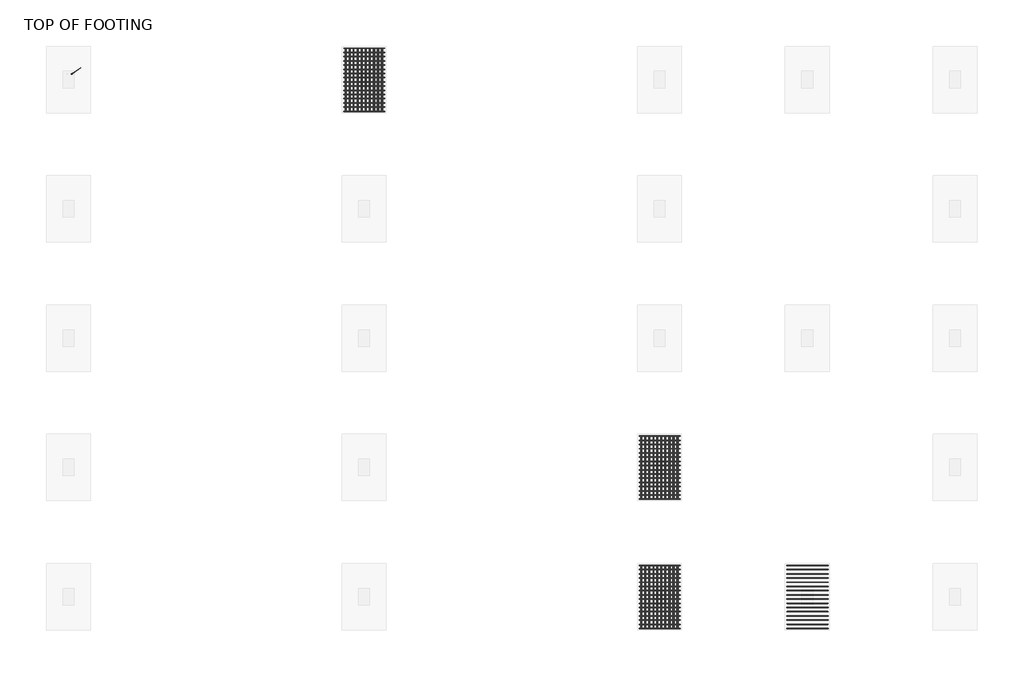
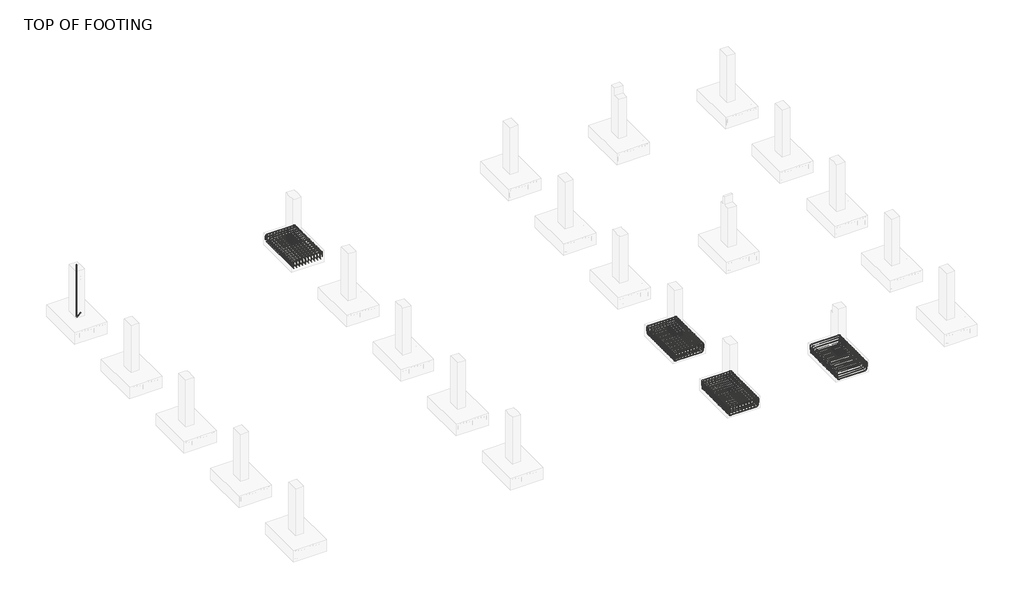
# One storey, part 5 of 8: 14 reinforcing bars.
"""IFC4 building model written with IfcOpenShell, lengths in millimetres."""

from ifc_helpers import new_model, si_unit, point, frame, origin, place, context, project, spatial, polyline, circle_curve, trimmed, segment, composite_curve, source, transform, mapped, element, save
from ifc_brep_helpers import swept_disk

model = new_model("IFC4")

# Units and contexts
model_context = context("Model", 3, world=origin())
ifc_project = project(units=[si_unit("LENGTHUNIT", "METRE", prefix="MILLI")], contexts=[model_context])

# Site, building, storey
site = spatial("IfcSite", under=ifc_project)
building = spatial("IfcBuilding", under=site)
storey = spatial("IfcBuildingStorey", under=building, Name="TOP OF FOOTING", Elevation=-1828.8)

# Reinforcing bars
placement = place(None, origin())
element("IfcReinforcingBar", 1, at=placement, inside=storey, context=model_context, shape_type="SolidModel", body=[
    swept_disk(composite_curve([segment(polyline([(-11755.8874017, 15924.2508557, -40.0), (-11755.8874017, 15924.2508557, -2055.5685723)]), True, "CONTINUOUS"), segment(trimmed(circle_curve(frame((-11717.9197045, 15950.8361235, -2055.5685723), z_axis=(0.5735764363510459, -0.819152044288992, 0.0), x_axis=(-37.96769719999975, -26.5852677999992, 0.0)), 46.35), [point((-11755.8874017, 15924.2508557, -2055.5685723))], [point((-11717.9197045, 15950.8361235, -2101.9185723))], True, "CARTESIAN"), True, "CONTINUOUS"), segment(polyline([(-11717.9197045, 15950.8361235, -2101.9185723), (-11506.0932621, 16099.1585953, -2101.9185723)]), True, "CONTINUOUS")], self_intersect=False), 6.35),
])
reinforcing_bar_shape = source(origin(), model_context, "Body", "SolidModel", [
    swept_disk(composite_curve([segment(polyline([(-4384.3374017, 16626.3508557, -2068.8), (-4384.3374017, 16626.3508557, -1921.5)]), True, "CONTINUOUS"), segment(trimmed(circle_curve(frame((-4337.9874017, 16626.3508557, -1921.5), z_axis=(0.0, 1.0, 0.0), x_axis=(-46.349999999999454, 0.0, 0.0)), 46.35), [point((-4384.3374017, 16626.3508557, -1921.5))], [point((-4337.9874017, 16626.3508557, -1875.15))], True, "CARTESIAN"), True, "CONTINUOUS"), segment(polyline([(-4337.9874017, 16626.3508557, -1875.15), (-3323.3874017, 16626.3508557, -1875.15)]), True, "CONTINUOUS"), segment(trimmed(circle_curve(frame((-3323.3874017, 16626.3508557, -1921.5), z_axis=(0.0, 1.0, 0.0), x_axis=(0.0, 0.0, 46.34999999999991)), 46.35), [point((-3323.3874017, 16626.3508557, -1875.15))], [point((-3277.0374017, 16626.3508557, -1921.5))], True, "CARTESIAN"), True, "CONTINUOUS"), segment(polyline([(-3277.0374017, 16626.3508557, -1921.5), (-3277.0374017, 16626.3508557, -2068.8)]), True, "CONTINUOUS")], self_intersect=False), 6.35),
])
element("IfcReinforcingBar", 2, at=placement, inside=storey, context=model_context, shape_type="MappedRepresentation", body=[
    mapped(reinforcing_bar_shape, transform((0.0, 0.0, 0.0), x_axis=(1.0, 0.0, 0.0), y_axis=(0.0, 1.0, 0.0), z_axis=(0.0, 0.0, 1.0))),
    mapped(reinforcing_bar_shape, transform((0.0, -113.82, 0.0), x_axis=(1.0, 0.0, 0.0), y_axis=(0.0, 1.0, 0.0), z_axis=(0.0, 0.0, 1.0))),
    mapped(reinforcing_bar_shape, transform((0.0, -227.64, 0.0), x_axis=(1.0, 0.0, 0.0), y_axis=(0.0, 1.0, 0.0), z_axis=(0.0, 0.0, 1.0))),
    mapped(reinforcing_bar_shape, transform((0.0, -341.46, 0.0), x_axis=(1.0, 0.0, 0.0), y_axis=(0.0, 1.0, 0.0), z_axis=(0.0, 0.0, 1.0))),
    mapped(reinforcing_bar_shape, transform((0.0, -455.28, 0.0), x_axis=(1.0, 0.0, 0.0), y_axis=(0.0, 1.0, 0.0), z_axis=(0.0, 0.0, 1.0))),
    mapped(reinforcing_bar_shape, transform((0.0, -569.1, 0.0), x_axis=(1.0, 0.0, 0.0), y_axis=(0.0, 1.0, 0.0), z_axis=(0.0, 0.0, 1.0))),
    mapped(reinforcing_bar_shape, transform((0.0, -682.92, 0.0), x_axis=(1.0, 0.0, 0.0), y_axis=(0.0, 1.0, 0.0), z_axis=(0.0, 0.0, 1.0))),
    mapped(reinforcing_bar_shape, transform((0.0, -796.74, 0.0), x_axis=(1.0, 0.0, 0.0), y_axis=(0.0, 1.0, 0.0), z_axis=(0.0, 0.0, 1.0))),
    mapped(reinforcing_bar_shape, transform((0.0, -910.56, 0.0), x_axis=(1.0, 0.0, 0.0), y_axis=(0.0, 1.0, 0.0), z_axis=(0.0, 0.0, 1.0))),
    mapped(reinforcing_bar_shape, transform((0.0, -1024.38, 0.0), x_axis=(1.0, 0.0, 0.0), y_axis=(0.0, 1.0, 0.0), z_axis=(0.0, 0.0, 1.0))),
    mapped(reinforcing_bar_shape, transform((0.0, -1138.2, 0.0), x_axis=(1.0, 0.0, 0.0), y_axis=(0.0, 1.0, 0.0), z_axis=(0.0, 0.0, 1.0))),
    mapped(reinforcing_bar_shape, transform((0.0, -1252.02, 0.0), x_axis=(1.0, 0.0, 0.0), y_axis=(0.0, 1.0, 0.0), z_axis=(0.0, 0.0, 1.0))),
    mapped(reinforcing_bar_shape, transform((0.0, -1365.84, 0.0), x_axis=(1.0, 0.0, 0.0), y_axis=(0.0, 1.0, 0.0), z_axis=(0.0, 0.0, 1.0))),
    mapped(reinforcing_bar_shape, transform((0.0, -1479.66, 0.0), x_axis=(1.0, 0.0, 0.0), y_axis=(0.0, 1.0, 0.0), z_axis=(0.0, 0.0, 1.0))),
    mapped(reinforcing_bar_shape, transform((0.0, -1593.48, 0.0), x_axis=(1.0, 0.0, 0.0), y_axis=(0.0, 1.0, 0.0), z_axis=(0.0, 0.0, 1.0))),
    mapped(reinforcing_bar_shape, transform((0.0, -1707.3, 0.0), x_axis=(1.0, 0.0, 0.0), y_axis=(0.0, 1.0, 0.0), z_axis=(0.0, 0.0, 1.0))),
])
reinforcing_bar_2_shape = source(origin(), model_context, "Body", "SolidModel", [
    swept_disk(composite_curve([segment(polyline([(-4339.592709, 16632.7008557, -2155.1176129), (-4339.592709, 14912.7008557, -2155.1176129)]), True, "CONTINUOUS")], self_intersect=False), 6.35),
])
element("IfcReinforcingBar", 3, at=placement, inside=storey, context=model_context, shape_type="MappedRepresentation", body=[
    mapped(reinforcing_bar_2_shape, transform((0.0, 0.0, 0.0), x_axis=(1.0, 0.0, 0.0), y_axis=(0.0, 1.0, 0.0), z_axis=(0.0, 0.0, 1.0))),
    mapped(reinforcing_bar_2_shape, transform((111.602188, 0.0, 0.0), x_axis=(1.0, 0.0, 0.0), y_axis=(0.0, 1.0, 0.0), z_axis=(0.0, 0.0, 1.0))),
    mapped(reinforcing_bar_2_shape, transform((223.2043759, 0.0, 0.0), x_axis=(1.0, 0.0, 0.0), y_axis=(0.0, 1.0, 0.0), z_axis=(0.0, 0.0, 1.0))),
    mapped(reinforcing_bar_2_shape, transform((334.8065639, 0.0, 0.0), x_axis=(1.0, 0.0, 0.0), y_axis=(0.0, 1.0, 0.0), z_axis=(0.0, 0.0, 1.0))),
    mapped(reinforcing_bar_2_shape, transform((446.4087519, 0.0, 0.0), x_axis=(1.0, 0.0, 0.0), y_axis=(0.0, 1.0, 0.0), z_axis=(0.0, 0.0, 1.0))),
    mapped(reinforcing_bar_2_shape, transform((558.0109398, 0.0, 0.0), x_axis=(1.0, 0.0, 0.0), y_axis=(0.0, 1.0, 0.0), z_axis=(0.0, 0.0, 1.0))),
    mapped(reinforcing_bar_2_shape, transform((669.6131278, 0.0, 0.0), x_axis=(1.0, 0.0, 0.0), y_axis=(0.0, 1.0, 0.0), z_axis=(0.0, 0.0, 1.0))),
    mapped(reinforcing_bar_2_shape, transform((781.2153158, 0.0, 0.0), x_axis=(1.0, 0.0, 0.0), y_axis=(0.0, 1.0, 0.0), z_axis=(0.0, 0.0, 1.0))),
    mapped(reinforcing_bar_2_shape, transform((892.8175037, 0.0, 0.0), x_axis=(1.0, 0.0, 0.0), y_axis=(0.0, 1.0, 0.0), z_axis=(0.0, 0.0, 1.0))),
    mapped(reinforcing_bar_2_shape, transform((1004.4196917, 0.0, 0.0), x_axis=(1.0, 0.0, 0.0), y_axis=(0.0, 1.0, 0.0), z_axis=(0.0, 0.0, 1.0))),
])
reinforcing_bar_3_shape = source(origin(), model_context, "Body", "SolidModel", [
    swept_disk(composite_curve([segment(polyline([(-3364.2651981, 16626.3508557, -2094.6521303), (-3364.2651981, 16626.3508557, -1947.3521303)]), True, "CONTINUOUS"), segment(trimmed(circle_curve(frame((-3364.2651981, 16580.0008557, -1947.3521303), z_axis=(1.0, 0.0, 0.0), x_axis=(0.0, 46.349999999998545, 0.0)), 46.35), [point((-3364.2651981, 16626.3508557, -1947.3521303))], [point((-3364.2651981, 16580.0008557, -1901.0021303))], True, "CARTESIAN"), True, "CONTINUOUS"), segment(polyline([(-3364.2651981, 16580.0008557, -1901.0021303), (-3364.2651981, 14965.4008557, -1901.0021303)]), True, "CONTINUOUS"), segment(trimmed(circle_curve(frame((-3364.2651981, 14965.4008557, -1947.3521303), z_axis=(1.0, 0.0, 0.0), x_axis=(0.0, 0.0, 46.34999999999991)), 46.35), [point((-3364.2651981, 14965.4008557, -1901.0021303))], [point((-3364.2651981, 14919.0508557, -1947.3521303))], True, "CARTESIAN"), True, "CONTINUOUS"), segment(polyline([(-3364.2651981, 14919.0508557, -1947.3521303), (-3364.2651981, 14919.0508557, -2094.6521303)]), True, "CONTINUOUS")], self_intersect=False), 6.35),
])
element("IfcReinforcingBar", 4, at=placement, inside=storey, context=model_context, shape_type="MappedRepresentation", body=[
    mapped(reinforcing_bar_3_shape, transform((0.0, 0.0, 0.0), x_axis=(1.0, 0.0, 0.0), y_axis=(0.0, 1.0, 0.0), z_axis=(0.0, 0.0, 1.0))),
    mapped(reinforcing_bar_3_shape, transform((-107.1680233, 0.0, 0.0), x_axis=(1.0, 0.0, 0.0), y_axis=(0.0, 1.0, 0.0), z_axis=(0.0, 0.0, 1.0))),
    mapped(reinforcing_bar_3_shape, transform((-214.3360466, 0.0, 0.0), x_axis=(1.0, 0.0, 0.0), y_axis=(0.0, 1.0, 0.0), z_axis=(0.0, 0.0, 1.0))),
    mapped(reinforcing_bar_3_shape, transform((-321.5040699, 0.0, 0.0), x_axis=(1.0, 0.0, 0.0), y_axis=(0.0, 1.0, 0.0), z_axis=(0.0, 0.0, 1.0))),
    mapped(reinforcing_bar_3_shape, transform((-428.6720932, 0.0, 0.0), x_axis=(1.0, 0.0, 0.0), y_axis=(0.0, 1.0, 0.0), z_axis=(0.0, 0.0, 1.0))),
    mapped(reinforcing_bar_3_shape, transform((-535.8401165, 0.0, 0.0), x_axis=(1.0, 0.0, 0.0), y_axis=(0.0, 1.0, 0.0), z_axis=(0.0, 0.0, 1.0))),
    mapped(reinforcing_bar_3_shape, transform((-643.0081398, 0.0, 0.0), x_axis=(1.0, 0.0, 0.0), y_axis=(0.0, 1.0, 0.0), z_axis=(0.0, 0.0, 1.0))),
    mapped(reinforcing_bar_3_shape, transform((-750.176163, 0.0, 0.0), x_axis=(1.0, 0.0, 0.0), y_axis=(0.0, 1.0, 0.0), z_axis=(0.0, 0.0, 1.0))),
    mapped(reinforcing_bar_3_shape, transform((-857.3441863, 0.0, 0.0), x_axis=(1.0, 0.0, 0.0), y_axis=(0.0, 1.0, 0.0), z_axis=(0.0, 0.0, 1.0))),
    mapped(reinforcing_bar_3_shape, transform((-964.5122096, 0.0, 0.0), x_axis=(1.0, 0.0, 0.0), y_axis=(0.0, 1.0, 0.0), z_axis=(0.0, 0.0, 1.0))),
])
reinforcing_bar_4_shape = source(origin(), model_context, "Body", "SolidModel", [
    swept_disk(composite_curve([segment(polyline([(4698.4779803, 2626.3508557, -2021.4413313), (4698.4779803, 2626.3508557, -2168.7413313)]), True, "CONTINUOUS"), segment(trimmed(circle_curve(frame((4652.1279803, 2626.3508557, -2168.7413313), z_axis=(0.0, 1.0, 0.0), x_axis=(46.350000000000364, 0.0, 0.0)), 46.35), [point((4698.4779803, 2626.3508557, -2168.7413313))], [point((4652.1279803, 2626.3508557, -2215.0913313))], True, "CARTESIAN"), True, "CONTINUOUS"), segment(polyline([(4652.1279803, 2626.3508557, -2215.0913313), (3679.832969, 2626.3508557, -2215.0913313)]), True, "CONTINUOUS"), segment(trimmed(circle_curve(frame((3679.832969, 2626.3508557, -2168.7413313), z_axis=(0.0, 1.0, 0.0), x_axis=(0.0, 0.0, -46.34999999999991)), 46.35), [point((3679.832969, 2626.3508557, -2215.0913313))], [point((3633.482969, 2626.3508557, -2168.7413313))], True, "CARTESIAN"), True, "CONTINUOUS"), segment(polyline([(3633.482969, 2626.3508557, -2168.7413313), (3633.482969, 2626.3508557, -2021.4413313)]), True, "CONTINUOUS")], self_intersect=False), 6.35),
])
element("IfcReinforcingBar", 5, at=placement, inside=storey, context=model_context, shape_type="MappedRepresentation", body=[
    mapped(reinforcing_bar_4_shape, transform((0.0, 0.0, 0.0), x_axis=(1.0, 0.0, 0.0), y_axis=(0.0, 1.0, 0.0), z_axis=(0.0, 0.0, 1.0))),
    mapped(reinforcing_bar_4_shape, transform((0.0, -113.82, 0.0), x_axis=(1.0, 0.0, 0.0), y_axis=(0.0, 1.0, 0.0), z_axis=(0.0, 0.0, 1.0))),
    mapped(reinforcing_bar_4_shape, transform((0.0, -227.64, 0.0), x_axis=(1.0, 0.0, 0.0), y_axis=(0.0, 1.0, 0.0), z_axis=(0.0, 0.0, 1.0))),
    mapped(reinforcing_bar_4_shape, transform((0.0, -341.46, 0.0), x_axis=(1.0, 0.0, 0.0), y_axis=(0.0, 1.0, 0.0), z_axis=(0.0, 0.0, 1.0))),
    mapped(reinforcing_bar_4_shape, transform((0.0, -455.28, 0.0), x_axis=(1.0, 0.0, 0.0), y_axis=(0.0, 1.0, 0.0), z_axis=(0.0, 0.0, 1.0))),
    mapped(reinforcing_bar_4_shape, transform((0.0, -569.1, 0.0), x_axis=(1.0, 0.0, 0.0), y_axis=(0.0, 1.0, 0.0), z_axis=(0.0, 0.0, 1.0))),
    mapped(reinforcing_bar_4_shape, transform((0.0, -682.92, 0.0), x_axis=(1.0, 0.0, 0.0), y_axis=(0.0, 1.0, 0.0), z_axis=(0.0, 0.0, 1.0))),
    mapped(reinforcing_bar_4_shape, transform((0.0, -796.74, 0.0), x_axis=(1.0, 0.0, 0.0), y_axis=(0.0, 1.0, 0.0), z_axis=(0.0, 0.0, 1.0))),
    mapped(reinforcing_bar_4_shape, transform((0.0, -910.56, 0.0), x_axis=(1.0, 0.0, 0.0), y_axis=(0.0, 1.0, 0.0), z_axis=(0.0, 0.0, 1.0))),
    mapped(reinforcing_bar_4_shape, transform((0.0, -1024.38, 0.0), x_axis=(1.0, 0.0, 0.0), y_axis=(0.0, 1.0, 0.0), z_axis=(0.0, 0.0, 1.0))),
    mapped(reinforcing_bar_4_shape, transform((0.0, -1138.2, 0.0), x_axis=(1.0, 0.0, 0.0), y_axis=(0.0, 1.0, 0.0), z_axis=(0.0, 0.0, 1.0))),
    mapped(reinforcing_bar_4_shape, transform((0.0, -1252.02, 0.0), x_axis=(1.0, 0.0, 0.0), y_axis=(0.0, 1.0, 0.0), z_axis=(0.0, 0.0, 1.0))),
    mapped(reinforcing_bar_4_shape, transform((0.0, -1365.84, 0.0), x_axis=(1.0, 0.0, 0.0), y_axis=(0.0, 1.0, 0.0), z_axis=(0.0, 0.0, 1.0))),
    mapped(reinforcing_bar_4_shape, transform((0.0, -1479.66, 0.0), x_axis=(1.0, 0.0, 0.0), y_axis=(0.0, 1.0, 0.0), z_axis=(0.0, 0.0, 1.0))),
    mapped(reinforcing_bar_4_shape, transform((0.0, -1593.48, 0.0), x_axis=(1.0, 0.0, 0.0), y_axis=(0.0, 1.0, 0.0), z_axis=(0.0, 0.0, 1.0))),
    mapped(reinforcing_bar_4_shape, transform((0.0, -1707.3, 0.0), x_axis=(1.0, 0.0, 0.0), y_axis=(0.0, 1.0, 0.0), z_axis=(0.0, 0.0, 1.0))),
])
reinforcing_bar_5_shape = source(origin(), model_context, "Body", "SolidModel", [
    swept_disk(composite_curve([segment(polyline([(3615.6625983, 2626.3508557, -2068.8), (3615.6625983, 2626.3508557, -1921.5)]), True, "CONTINUOUS"), segment(trimmed(circle_curve(frame((3662.0125983, 2626.3508557, -1921.5), z_axis=(0.0, 1.0, 0.0), x_axis=(-46.34999999999991, 0.0, 0.0)), 46.35), [point((3615.6625983, 2626.3508557, -1921.5))], [point((3662.0125983, 2626.3508557, -1875.15))], True, "CARTESIAN"), True, "CONTINUOUS"), segment(polyline([(3662.0125983, 2626.3508557, -1875.15), (4676.6125983, 2626.3508557, -1875.15)]), True, "CONTINUOUS"), segment(trimmed(circle_curve(frame((4676.6125983, 2626.3508557, -1921.5), z_axis=(0.0, 1.0, 0.0), x_axis=(0.0, 0.0, 46.34999999999991)), 46.35), [point((4676.6125983, 2626.3508557, -1875.15))], [point((4722.9625983, 2626.3508557, -1921.5))], True, "CARTESIAN"), True, "CONTINUOUS"), segment(polyline([(4722.9625983, 2626.3508557, -1921.5), (4722.9625983, 2626.3508557, -2068.8)]), True, "CONTINUOUS")], self_intersect=False), 6.35),
])
element("IfcReinforcingBar", 6, at=placement, inside=storey, context=model_context, shape_type="MappedRepresentation", body=[
    mapped(reinforcing_bar_5_shape, transform((0.0, 0.0, 0.0), x_axis=(1.0, 0.0, 0.0), y_axis=(0.0, 1.0, 0.0), z_axis=(0.0, 0.0, 1.0))),
    mapped(reinforcing_bar_5_shape, transform((0.0, -113.82, 0.0), x_axis=(1.0, 0.0, 0.0), y_axis=(0.0, 1.0, 0.0), z_axis=(0.0, 0.0, 1.0))),
    mapped(reinforcing_bar_5_shape, transform((0.0, -227.64, 0.0), x_axis=(1.0, 0.0, 0.0), y_axis=(0.0, 1.0, 0.0), z_axis=(0.0, 0.0, 1.0))),
    mapped(reinforcing_bar_5_shape, transform((0.0, -341.46, 0.0), x_axis=(1.0, 0.0, 0.0), y_axis=(0.0, 1.0, 0.0), z_axis=(0.0, 0.0, 1.0))),
    mapped(reinforcing_bar_5_shape, transform((0.0, -455.28, 0.0), x_axis=(1.0, 0.0, 0.0), y_axis=(0.0, 1.0, 0.0), z_axis=(0.0, 0.0, 1.0))),
    mapped(reinforcing_bar_5_shape, transform((0.0, -569.1, 0.0), x_axis=(1.0, 0.0, 0.0), y_axis=(0.0, 1.0, 0.0), z_axis=(0.0, 0.0, 1.0))),
    mapped(reinforcing_bar_5_shape, transform((0.0, -682.92, 0.0), x_axis=(1.0, 0.0, 0.0), y_axis=(0.0, 1.0, 0.0), z_axis=(0.0, 0.0, 1.0))),
    mapped(reinforcing_bar_5_shape, transform((0.0, -796.74, 0.0), x_axis=(1.0, 0.0, 0.0), y_axis=(0.0, 1.0, 0.0), z_axis=(0.0, 0.0, 1.0))),
    mapped(reinforcing_bar_5_shape, transform((0.0, -910.56, 0.0), x_axis=(1.0, 0.0, 0.0), y_axis=(0.0, 1.0, 0.0), z_axis=(0.0, 0.0, 1.0))),
    mapped(reinforcing_bar_5_shape, transform((0.0, -1024.38, 0.0), x_axis=(1.0, 0.0, 0.0), y_axis=(0.0, 1.0, 0.0), z_axis=(0.0, 0.0, 1.0))),
    mapped(reinforcing_bar_5_shape, transform((0.0, -1138.2, 0.0), x_axis=(1.0, 0.0, 0.0), y_axis=(0.0, 1.0, 0.0), z_axis=(0.0, 0.0, 1.0))),
    mapped(reinforcing_bar_5_shape, transform((0.0, -1252.02, 0.0), x_axis=(1.0, 0.0, 0.0), y_axis=(0.0, 1.0, 0.0), z_axis=(0.0, 0.0, 1.0))),
    mapped(reinforcing_bar_5_shape, transform((0.0, -1365.84, 0.0), x_axis=(1.0, 0.0, 0.0), y_axis=(0.0, 1.0, 0.0), z_axis=(0.0, 0.0, 1.0))),
    mapped(reinforcing_bar_5_shape, transform((0.0, -1479.66, 0.0), x_axis=(1.0, 0.0, 0.0), y_axis=(0.0, 1.0, 0.0), z_axis=(0.0, 0.0, 1.0))),
    mapped(reinforcing_bar_5_shape, transform((0.0, -1593.48, 0.0), x_axis=(1.0, 0.0, 0.0), y_axis=(0.0, 1.0, 0.0), z_axis=(0.0, 0.0, 1.0))),
    mapped(reinforcing_bar_5_shape, transform((0.0, -1707.3, 0.0), x_axis=(1.0, 0.0, 0.0), y_axis=(0.0, 1.0, 0.0), z_axis=(0.0, 0.0, 1.0))),
])
reinforcing_bar_6_shape = source(origin(), model_context, "Body", "SolidModel", [
    swept_disk(composite_curve([segment(polyline([(3660.407291, 2632.7008557, -2155.1176129), (3660.407291, 912.7008557, -2155.1176129)]), True, "CONTINUOUS")], self_intersect=False), 6.35),
])
element("IfcReinforcingBar", 7, at=placement, inside=storey, context=model_context, shape_type="MappedRepresentation", body=[
    mapped(reinforcing_bar_6_shape, transform((0.0, 0.0, 0.0), x_axis=(1.0, 0.0, 0.0), y_axis=(0.0, 1.0, 0.0), z_axis=(0.0, 0.0, 1.0))),
    mapped(reinforcing_bar_6_shape, transform((111.602188, 0.0, 0.0), x_axis=(1.0, 0.0, 0.0), y_axis=(0.0, 1.0, 0.0), z_axis=(0.0, 0.0, 1.0))),
    mapped(reinforcing_bar_6_shape, transform((223.2043759, 0.0, 0.0), x_axis=(1.0, 0.0, 0.0), y_axis=(0.0, 1.0, 0.0), z_axis=(0.0, 0.0, 1.0))),
    mapped(reinforcing_bar_6_shape, transform((334.8065639, 0.0, 0.0), x_axis=(1.0, 0.0, 0.0), y_axis=(0.0, 1.0, 0.0), z_axis=(0.0, 0.0, 1.0))),
    mapped(reinforcing_bar_6_shape, transform((446.4087519, 0.0, 0.0), x_axis=(1.0, 0.0, 0.0), y_axis=(0.0, 1.0, 0.0), z_axis=(0.0, 0.0, 1.0))),
    mapped(reinforcing_bar_6_shape, transform((558.0109398, 0.0, 0.0), x_axis=(1.0, 0.0, 0.0), y_axis=(0.0, 1.0, 0.0), z_axis=(0.0, 0.0, 1.0))),
    mapped(reinforcing_bar_6_shape, transform((669.6131278, 0.0, 0.0), x_axis=(1.0, 0.0, 0.0), y_axis=(0.0, 1.0, 0.0), z_axis=(0.0, 0.0, 1.0))),
    mapped(reinforcing_bar_6_shape, transform((781.2153158, 0.0, 0.0), x_axis=(1.0, 0.0, 0.0), y_axis=(0.0, 1.0, 0.0), z_axis=(0.0, 0.0, 1.0))),
    mapped(reinforcing_bar_6_shape, transform((892.8175037, 0.0, 0.0), x_axis=(1.0, 0.0, 0.0), y_axis=(0.0, 1.0, 0.0), z_axis=(0.0, 0.0, 1.0))),
    mapped(reinforcing_bar_6_shape, transform((1004.4196917, 0.0, 0.0), x_axis=(1.0, 0.0, 0.0), y_axis=(0.0, 1.0, 0.0), z_axis=(0.0, 0.0, 1.0))),
])
reinforcing_bar_7_shape = source(origin(), model_context, "Body", "SolidModel", [
    swept_disk(composite_curve([segment(polyline([(4635.7348019, 2626.3508557, -2094.6521303), (4635.7348019, 2626.3508557, -1947.3521303)]), True, "CONTINUOUS"), segment(trimmed(circle_curve(frame((4635.7348019, 2580.0008557, -1947.3521303), z_axis=(1.0, 0.0, 0.0), x_axis=(0.0, 46.34999999999991, 0.0)), 46.35), [point((4635.7348019, 2626.3508557, -1947.3521303))], [point((4635.7348019, 2580.0008557, -1901.0021303))], True, "CARTESIAN"), True, "CONTINUOUS"), segment(polyline([(4635.7348019, 2580.0008557, -1901.0021303), (4635.7348019, 965.4008557, -1901.0021303)]), True, "CONTINUOUS"), segment(trimmed(circle_curve(frame((4635.7348019, 965.4008557, -1947.3521303), z_axis=(1.0, 0.0, 0.0), x_axis=(0.0, 0.0, 46.34999999999991)), 46.35), [point((4635.7348019, 965.4008557, -1901.0021303))], [point((4635.7348019, 919.0508557, -1947.3521303))], True, "CARTESIAN"), True, "CONTINUOUS"), segment(polyline([(4635.7348019, 919.0508557, -1947.3521303), (4635.7348019, 919.0508557, -2094.6521303)]), True, "CONTINUOUS")], self_intersect=False), 6.35),
])
element("IfcReinforcingBar", 8, at=placement, inside=storey, context=model_context, shape_type="MappedRepresentation", body=[
    mapped(reinforcing_bar_7_shape, transform((0.0, 0.0, 0.0), x_axis=(1.0, 0.0, 0.0), y_axis=(0.0, 1.0, 0.0), z_axis=(0.0, 0.0, 1.0))),
    mapped(reinforcing_bar_7_shape, transform((-107.1680233, 0.0, 0.0), x_axis=(1.0, 0.0, 0.0), y_axis=(0.0, 1.0, 0.0), z_axis=(0.0, 0.0, 1.0))),
    mapped(reinforcing_bar_7_shape, transform((-214.3360466, 0.0, 0.0), x_axis=(1.0, 0.0, 0.0), y_axis=(0.0, 1.0, 0.0), z_axis=(0.0, 0.0, 1.0))),
    mapped(reinforcing_bar_7_shape, transform((-321.5040699, 0.0, 0.0), x_axis=(1.0, 0.0, 0.0), y_axis=(0.0, 1.0, 0.0), z_axis=(0.0, 0.0, 1.0))),
    mapped(reinforcing_bar_7_shape, transform((-428.6720932, 0.0, 0.0), x_axis=(1.0, 0.0, 0.0), y_axis=(0.0, 1.0, 0.0), z_axis=(0.0, 0.0, 1.0))),
    mapped(reinforcing_bar_7_shape, transform((-535.8401165, 0.0, 0.0), x_axis=(1.0, 0.0, 0.0), y_axis=(0.0, 1.0, 0.0), z_axis=(0.0, 0.0, 1.0))),
    mapped(reinforcing_bar_7_shape, transform((-643.0081398, 0.0, 0.0), x_axis=(1.0, 0.0, 0.0), y_axis=(0.0, 1.0, 0.0), z_axis=(0.0, 0.0, 1.0))),
    mapped(reinforcing_bar_7_shape, transform((-750.176163, 0.0, 0.0), x_axis=(1.0, 0.0, 0.0), y_axis=(0.0, 1.0, 0.0), z_axis=(0.0, 0.0, 1.0))),
    mapped(reinforcing_bar_7_shape, transform((-857.3441863, 0.0, 0.0), x_axis=(1.0, 0.0, 0.0), y_axis=(0.0, 1.0, 0.0), z_axis=(0.0, 0.0, 1.0))),
    mapped(reinforcing_bar_7_shape, transform((-964.5122096, 0.0, 0.0), x_axis=(1.0, 0.0, 0.0), y_axis=(0.0, 1.0, 0.0), z_axis=(0.0, 0.0, 1.0))),
])
reinforcing_bar_8_shape = source(origin(), model_context, "Body", "SolidModel", [
    swept_disk(composite_curve([segment(polyline([(4698.4779803, 6126.3508557, -2021.4413313), (4698.4779803, 6126.3508557, -2168.7413313)]), True, "CONTINUOUS"), segment(trimmed(circle_curve(frame((4652.1279803, 6126.3508557, -2168.7413313), z_axis=(0.0, 1.0, 0.0), x_axis=(46.350000000000364, 0.0, 0.0)), 46.35), [point((4698.4779803, 6126.3508557, -2168.7413313))], [point((4652.1279803, 6126.3508557, -2215.0913313))], True, "CARTESIAN"), True, "CONTINUOUS"), segment(polyline([(4652.1279803, 6126.3508557, -2215.0913313), (3679.832969, 6126.3508557, -2215.0913313)]), True, "CONTINUOUS"), segment(trimmed(circle_curve(frame((3679.832969, 6126.3508557, -2168.7413313), z_axis=(0.0, 1.0, 0.0), x_axis=(0.0, 0.0, -46.34999999999991)), 46.35), [point((3679.832969, 6126.3508557, -2215.0913313))], [point((3633.482969, 6126.3508557, -2168.7413313))], True, "CARTESIAN"), True, "CONTINUOUS"), segment(polyline([(3633.482969, 6126.3508557, -2168.7413313), (3633.482969, 6126.3508557, -2021.4413313)]), True, "CONTINUOUS")], self_intersect=False), 6.35),
])
element("IfcReinforcingBar", 9, at=placement, inside=storey, context=model_context, shape_type="MappedRepresentation", body=[
    mapped(reinforcing_bar_8_shape, transform((0.0, 0.0, 0.0), x_axis=(1.0, 0.0, 0.0), y_axis=(0.0, 1.0, 0.0), z_axis=(0.0, 0.0, 1.0))),
    mapped(reinforcing_bar_8_shape, transform((0.0, -113.82, 0.0), x_axis=(1.0, 0.0, 0.0), y_axis=(0.0, 1.0, 0.0), z_axis=(0.0, 0.0, 1.0))),
    mapped(reinforcing_bar_8_shape, transform((0.0, -227.64, 0.0), x_axis=(1.0, 0.0, 0.0), y_axis=(0.0, 1.0, 0.0), z_axis=(0.0, 0.0, 1.0))),
    mapped(reinforcing_bar_8_shape, transform((0.0, -341.46, 0.0), x_axis=(1.0, 0.0, 0.0), y_axis=(0.0, 1.0, 0.0), z_axis=(0.0, 0.0, 1.0))),
    mapped(reinforcing_bar_8_shape, transform((0.0, -455.28, 0.0), x_axis=(1.0, 0.0, 0.0), y_axis=(0.0, 1.0, 0.0), z_axis=(0.0, 0.0, 1.0))),
    mapped(reinforcing_bar_8_shape, transform((0.0, -569.1, 0.0), x_axis=(1.0, 0.0, 0.0), y_axis=(0.0, 1.0, 0.0), z_axis=(0.0, 0.0, 1.0))),
    mapped(reinforcing_bar_8_shape, transform((0.0, -682.92, 0.0), x_axis=(1.0, 0.0, 0.0), y_axis=(0.0, 1.0, 0.0), z_axis=(0.0, 0.0, 1.0))),
    mapped(reinforcing_bar_8_shape, transform((0.0, -796.74, 0.0), x_axis=(1.0, 0.0, 0.0), y_axis=(0.0, 1.0, 0.0), z_axis=(0.0, 0.0, 1.0))),
    mapped(reinforcing_bar_8_shape, transform((0.0, -910.56, 0.0), x_axis=(1.0, 0.0, 0.0), y_axis=(0.0, 1.0, 0.0), z_axis=(0.0, 0.0, 1.0))),
    mapped(reinforcing_bar_8_shape, transform((0.0, -1024.38, 0.0), x_axis=(1.0, 0.0, 0.0), y_axis=(0.0, 1.0, 0.0), z_axis=(0.0, 0.0, 1.0))),
    mapped(reinforcing_bar_8_shape, transform((0.0, -1138.2, 0.0), x_axis=(1.0, 0.0, 0.0), y_axis=(0.0, 1.0, 0.0), z_axis=(0.0, 0.0, 1.0))),
    mapped(reinforcing_bar_8_shape, transform((0.0, -1252.02, 0.0), x_axis=(1.0, 0.0, 0.0), y_axis=(0.0, 1.0, 0.0), z_axis=(0.0, 0.0, 1.0))),
    mapped(reinforcing_bar_8_shape, transform((0.0, -1365.84, 0.0), x_axis=(1.0, 0.0, 0.0), y_axis=(0.0, 1.0, 0.0), z_axis=(0.0, 0.0, 1.0))),
    mapped(reinforcing_bar_8_shape, transform((0.0, -1479.66, 0.0), x_axis=(1.0, 0.0, 0.0), y_axis=(0.0, 1.0, 0.0), z_axis=(0.0, 0.0, 1.0))),
    mapped(reinforcing_bar_8_shape, transform((0.0, -1593.48, 0.0), x_axis=(1.0, 0.0, 0.0), y_axis=(0.0, 1.0, 0.0), z_axis=(0.0, 0.0, 1.0))),
    mapped(reinforcing_bar_8_shape, transform((0.0, -1707.3, 0.0), x_axis=(1.0, 0.0, 0.0), y_axis=(0.0, 1.0, 0.0), z_axis=(0.0, 0.0, 1.0))),
])
reinforcing_bar_9_shape = source(origin(), model_context, "Body", "SolidModel", [
    swept_disk(composite_curve([segment(polyline([(3615.6625983, 6126.3508557, -2068.8), (3615.6625983, 6126.3508557, -1921.5)]), True, "CONTINUOUS"), segment(trimmed(circle_curve(frame((3662.0125983, 6126.3508557, -1921.5), z_axis=(0.0, 1.0, 0.0), x_axis=(-46.34999999999991, 0.0, 0.0)), 46.35), [point((3615.6625983, 6126.3508557, -1921.5))], [point((3662.0125983, 6126.3508557, -1875.15))], True, "CARTESIAN"), True, "CONTINUOUS"), segment(polyline([(3662.0125983, 6126.3508557, -1875.15), (4676.6125983, 6126.3508557, -1875.15)]), True, "CONTINUOUS"), segment(trimmed(circle_curve(frame((4676.6125983, 6126.3508557, -1921.5), z_axis=(0.0, 1.0, 0.0), x_axis=(0.0, 0.0, 46.34999999999991)), 46.35), [point((4676.6125983, 6126.3508557, -1875.15))], [point((4722.9625983, 6126.3508557, -1921.5))], True, "CARTESIAN"), True, "CONTINUOUS"), segment(polyline([(4722.9625983, 6126.3508557, -1921.5), (4722.9625983, 6126.3508557, -2068.8)]), True, "CONTINUOUS")], self_intersect=False), 6.35),
])
element("IfcReinforcingBar", 10, at=placement, inside=storey, context=model_context, shape_type="MappedRepresentation", body=[
    mapped(reinforcing_bar_9_shape, transform((0.0, 0.0, 0.0), x_axis=(1.0, 0.0, 0.0), y_axis=(0.0, 1.0, 0.0), z_axis=(0.0, 0.0, 1.0))),
    mapped(reinforcing_bar_9_shape, transform((0.0, -113.82, 0.0), x_axis=(1.0, 0.0, 0.0), y_axis=(0.0, 1.0, 0.0), z_axis=(0.0, 0.0, 1.0))),
    mapped(reinforcing_bar_9_shape, transform((0.0, -227.64, 0.0), x_axis=(1.0, 0.0, 0.0), y_axis=(0.0, 1.0, 0.0), z_axis=(0.0, 0.0, 1.0))),
    mapped(reinforcing_bar_9_shape, transform((0.0, -341.46, 0.0), x_axis=(1.0, 0.0, 0.0), y_axis=(0.0, 1.0, 0.0), z_axis=(0.0, 0.0, 1.0))),
    mapped(reinforcing_bar_9_shape, transform((0.0, -455.28, 0.0), x_axis=(1.0, 0.0, 0.0), y_axis=(0.0, 1.0, 0.0), z_axis=(0.0, 0.0, 1.0))),
    mapped(reinforcing_bar_9_shape, transform((0.0, -569.1, 0.0), x_axis=(1.0, 0.0, 0.0), y_axis=(0.0, 1.0, 0.0), z_axis=(0.0, 0.0, 1.0))),
    mapped(reinforcing_bar_9_shape, transform((0.0, -682.92, 0.0), x_axis=(1.0, 0.0, 0.0), y_axis=(0.0, 1.0, 0.0), z_axis=(0.0, 0.0, 1.0))),
    mapped(reinforcing_bar_9_shape, transform((0.0, -796.74, 0.0), x_axis=(1.0, 0.0, 0.0), y_axis=(0.0, 1.0, 0.0), z_axis=(0.0, 0.0, 1.0))),
    mapped(reinforcing_bar_9_shape, transform((0.0, -910.56, 0.0), x_axis=(1.0, 0.0, 0.0), y_axis=(0.0, 1.0, 0.0), z_axis=(0.0, 0.0, 1.0))),
    mapped(reinforcing_bar_9_shape, transform((0.0, -1024.38, 0.0), x_axis=(1.0, 0.0, 0.0), y_axis=(0.0, 1.0, 0.0), z_axis=(0.0, 0.0, 1.0))),
    mapped(reinforcing_bar_9_shape, transform((0.0, -1138.2, 0.0), x_axis=(1.0, 0.0, 0.0), y_axis=(0.0, 1.0, 0.0), z_axis=(0.0, 0.0, 1.0))),
    mapped(reinforcing_bar_9_shape, transform((0.0, -1252.02, 0.0), x_axis=(1.0, 0.0, 0.0), y_axis=(0.0, 1.0, 0.0), z_axis=(0.0, 0.0, 1.0))),
    mapped(reinforcing_bar_9_shape, transform((0.0, -1365.84, 0.0), x_axis=(1.0, 0.0, 0.0), y_axis=(0.0, 1.0, 0.0), z_axis=(0.0, 0.0, 1.0))),
    mapped(reinforcing_bar_9_shape, transform((0.0, -1479.66, 0.0), x_axis=(1.0, 0.0, 0.0), y_axis=(0.0, 1.0, 0.0), z_axis=(0.0, 0.0, 1.0))),
    mapped(reinforcing_bar_9_shape, transform((0.0, -1593.48, 0.0), x_axis=(1.0, 0.0, 0.0), y_axis=(0.0, 1.0, 0.0), z_axis=(0.0, 0.0, 1.0))),
    mapped(reinforcing_bar_9_shape, transform((0.0, -1707.3, 0.0), x_axis=(1.0, 0.0, 0.0), y_axis=(0.0, 1.0, 0.0), z_axis=(0.0, 0.0, 1.0))),
])
reinforcing_bar_10_shape = source(origin(), model_context, "Body", "SolidModel", [
    swept_disk(composite_curve([segment(polyline([(3660.407291, 6132.7008557, -2155.1176129), (3660.407291, 4412.7008557, -2155.1176129)]), True, "CONTINUOUS")], self_intersect=False), 6.35),
])
element("IfcReinforcingBar", 11, at=placement, inside=storey, context=model_context, shape_type="MappedRepresentation", body=[
    mapped(reinforcing_bar_10_shape, transform((0.0, 0.0, 0.0), x_axis=(1.0, 0.0, 0.0), y_axis=(0.0, 1.0, 0.0), z_axis=(0.0, 0.0, 1.0))),
    mapped(reinforcing_bar_10_shape, transform((111.602188, 0.0, 0.0), x_axis=(1.0, 0.0, 0.0), y_axis=(0.0, 1.0, 0.0), z_axis=(0.0, 0.0, 1.0))),
    mapped(reinforcing_bar_10_shape, transform((223.2043759, 0.0, 0.0), x_axis=(1.0, 0.0, 0.0), y_axis=(0.0, 1.0, 0.0), z_axis=(0.0, 0.0, 1.0))),
    mapped(reinforcing_bar_10_shape, transform((334.8065639, 0.0, 0.0), x_axis=(1.0, 0.0, 0.0), y_axis=(0.0, 1.0, 0.0), z_axis=(0.0, 0.0, 1.0))),
    mapped(reinforcing_bar_10_shape, transform((446.4087519, 0.0, 0.0), x_axis=(1.0, 0.0, 0.0), y_axis=(0.0, 1.0, 0.0), z_axis=(0.0, 0.0, 1.0))),
    mapped(reinforcing_bar_10_shape, transform((558.0109398, 0.0, 0.0), x_axis=(1.0, 0.0, 0.0), y_axis=(0.0, 1.0, 0.0), z_axis=(0.0, 0.0, 1.0))),
    mapped(reinforcing_bar_10_shape, transform((669.6131278, 0.0, 0.0), x_axis=(1.0, 0.0, 0.0), y_axis=(0.0, 1.0, 0.0), z_axis=(0.0, 0.0, 1.0))),
    mapped(reinforcing_bar_10_shape, transform((781.2153158, 0.0, 0.0), x_axis=(1.0, 0.0, 0.0), y_axis=(0.0, 1.0, 0.0), z_axis=(0.0, 0.0, 1.0))),
    mapped(reinforcing_bar_10_shape, transform((892.8175037, 0.0, 0.0), x_axis=(1.0, 0.0, 0.0), y_axis=(0.0, 1.0, 0.0), z_axis=(0.0, 0.0, 1.0))),
    mapped(reinforcing_bar_10_shape, transform((1004.4196917, 0.0, 0.0), x_axis=(1.0, 0.0, 0.0), y_axis=(0.0, 1.0, 0.0), z_axis=(0.0, 0.0, 1.0))),
])
reinforcing_bar_11_shape = source(origin(), model_context, "Body", "SolidModel", [
    swept_disk(composite_curve([segment(polyline([(4635.7348019, 6126.3508557, -2094.6521303), (4635.7348019, 6126.3508557, -1947.3521303)]), True, "CONTINUOUS"), segment(trimmed(circle_curve(frame((4635.7348019, 6080.0008557, -1947.3521303), z_axis=(1.0, 0.0, 0.0), x_axis=(0.0, 46.349999999999454, 0.0)), 46.35), [point((4635.7348019, 6126.3508557, -1947.3521303))], [point((4635.7348019, 6080.0008557, -1901.0021303))], True, "CARTESIAN"), True, "CONTINUOUS"), segment(polyline([(4635.7348019, 6080.0008557, -1901.0021303), (4635.7348019, 4465.4008557, -1901.0021303)]), True, "CONTINUOUS"), segment(trimmed(circle_curve(frame((4635.7348019, 4465.4008557, -1947.3521303), z_axis=(1.0, 0.0, 0.0), x_axis=(0.0, 0.0, 46.34999999999991)), 46.35), [point((4635.7348019, 4465.4008557, -1901.0021303))], [point((4635.7348019, 4419.0508557, -1947.3521303))], True, "CARTESIAN"), True, "CONTINUOUS"), segment(polyline([(4635.7348019, 4419.0508557, -1947.3521303), (4635.7348019, 4419.0508557, -2094.6521303)]), True, "CONTINUOUS")], self_intersect=False), 6.35),
])
element("IfcReinforcingBar", 12, at=placement, inside=storey, context=model_context, shape_type="MappedRepresentation", body=[
    mapped(reinforcing_bar_11_shape, transform((0.0, 0.0, 0.0), x_axis=(1.0, 0.0, 0.0), y_axis=(0.0, 1.0, 0.0), z_axis=(0.0, 0.0, 1.0))),
    mapped(reinforcing_bar_11_shape, transform((-107.1680233, 0.0, 0.0), x_axis=(1.0, 0.0, 0.0), y_axis=(0.0, 1.0, 0.0), z_axis=(0.0, 0.0, 1.0))),
    mapped(reinforcing_bar_11_shape, transform((-214.3360466, 0.0, 0.0), x_axis=(1.0, 0.0, 0.0), y_axis=(0.0, 1.0, 0.0), z_axis=(0.0, 0.0, 1.0))),
    mapped(reinforcing_bar_11_shape, transform((-321.5040699, 0.0, 0.0), x_axis=(1.0, 0.0, 0.0), y_axis=(0.0, 1.0, 0.0), z_axis=(0.0, 0.0, 1.0))),
    mapped(reinforcing_bar_11_shape, transform((-428.6720932, 0.0, 0.0), x_axis=(1.0, 0.0, 0.0), y_axis=(0.0, 1.0, 0.0), z_axis=(0.0, 0.0, 1.0))),
    mapped(reinforcing_bar_11_shape, transform((-535.8401165, 0.0, 0.0), x_axis=(1.0, 0.0, 0.0), y_axis=(0.0, 1.0, 0.0), z_axis=(0.0, 0.0, 1.0))),
    mapped(reinforcing_bar_11_shape, transform((-643.0081398, 0.0, 0.0), x_axis=(1.0, 0.0, 0.0), y_axis=(0.0, 1.0, 0.0), z_axis=(0.0, 0.0, 1.0))),
    mapped(reinforcing_bar_11_shape, transform((-750.176163, 0.0, 0.0), x_axis=(1.0, 0.0, 0.0), y_axis=(0.0, 1.0, 0.0), z_axis=(0.0, 0.0, 1.0))),
    mapped(reinforcing_bar_11_shape, transform((-857.3441863, 0.0, 0.0), x_axis=(1.0, 0.0, 0.0), y_axis=(0.0, 1.0, 0.0), z_axis=(0.0, 0.0, 1.0))),
    mapped(reinforcing_bar_11_shape, transform((-964.5122096, 0.0, 0.0), x_axis=(1.0, 0.0, 0.0), y_axis=(0.0, 1.0, 0.0), z_axis=(0.0, 0.0, 1.0))),
])
reinforcing_bar_12_shape = source(origin(), model_context, "Body", "SolidModel", [
    swept_disk(composite_curve([segment(polyline([(8698.4779803, 2626.3508557, -2021.4413313), (8698.4779803, 2626.3508557, -2168.7413313)]), True, "CONTINUOUS"), segment(trimmed(circle_curve(frame((8652.1279803, 2626.3508557, -2168.7413313), z_axis=(0.0, 1.0, 0.0), x_axis=(46.350000000000364, 0.0, 0.0)), 46.35), [point((8698.4779803, 2626.3508557, -2168.7413313))], [point((8652.1279803, 2626.3508557, -2215.0913313))], True, "CARTESIAN"), True, "CONTINUOUS"), segment(polyline([(8652.1279803, 2626.3508557, -2215.0913313), (7679.832969, 2626.3508557, -2215.0913313)]), True, "CONTINUOUS"), segment(trimmed(circle_curve(frame((7679.832969, 2626.3508557, -2168.7413313), z_axis=(0.0, 1.0, 0.0), x_axis=(0.0, 0.0, -46.34999999999991)), 46.35), [point((7679.832969, 2626.3508557, -2215.0913313))], [point((7633.482969, 2626.3508557, -2168.7413313))], True, "CARTESIAN"), True, "CONTINUOUS"), segment(polyline([(7633.482969, 2626.3508557, -2168.7413313), (7633.482969, 2626.3508557, -2021.4413313)]), True, "CONTINUOUS")], self_intersect=False), 6.35),
])
element("IfcReinforcingBar", 13, at=placement, inside=storey, context=model_context, shape_type="MappedRepresentation", body=[
    mapped(reinforcing_bar_12_shape, transform((0.0, 0.0, 0.0), x_axis=(1.0, 0.0, 0.0), y_axis=(0.0, 1.0, 0.0), z_axis=(0.0, 0.0, 1.0))),
    mapped(reinforcing_bar_12_shape, transform((0.0, -113.82, 0.0), x_axis=(1.0, 0.0, 0.0), y_axis=(0.0, 1.0, 0.0), z_axis=(0.0, 0.0, 1.0))),
    mapped(reinforcing_bar_12_shape, transform((0.0, -227.64, 0.0), x_axis=(1.0, 0.0, 0.0), y_axis=(0.0, 1.0, 0.0), z_axis=(0.0, 0.0, 1.0))),
    mapped(reinforcing_bar_12_shape, transform((0.0, -341.46, 0.0), x_axis=(1.0, 0.0, 0.0), y_axis=(0.0, 1.0, 0.0), z_axis=(0.0, 0.0, 1.0))),
    mapped(reinforcing_bar_12_shape, transform((0.0, -455.28, 0.0), x_axis=(1.0, 0.0, 0.0), y_axis=(0.0, 1.0, 0.0), z_axis=(0.0, 0.0, 1.0))),
    mapped(reinforcing_bar_12_shape, transform((0.0, -569.1, 0.0), x_axis=(1.0, 0.0, 0.0), y_axis=(0.0, 1.0, 0.0), z_axis=(0.0, 0.0, 1.0))),
    mapped(reinforcing_bar_12_shape, transform((0.0, -682.92, 0.0), x_axis=(1.0, 0.0, 0.0), y_axis=(0.0, 1.0, 0.0), z_axis=(0.0, 0.0, 1.0))),
    mapped(reinforcing_bar_12_shape, transform((0.0, -796.74, 0.0), x_axis=(1.0, 0.0, 0.0), y_axis=(0.0, 1.0, 0.0), z_axis=(0.0, 0.0, 1.0))),
    mapped(reinforcing_bar_12_shape, transform((0.0, -910.56, 0.0), x_axis=(1.0, 0.0, 0.0), y_axis=(0.0, 1.0, 0.0), z_axis=(0.0, 0.0, 1.0))),
    mapped(reinforcing_bar_12_shape, transform((0.0, -1024.38, 0.0), x_axis=(1.0, 0.0, 0.0), y_axis=(0.0, 1.0, 0.0), z_axis=(0.0, 0.0, 1.0))),
    mapped(reinforcing_bar_12_shape, transform((0.0, -1138.2, 0.0), x_axis=(1.0, 0.0, 0.0), y_axis=(0.0, 1.0, 0.0), z_axis=(0.0, 0.0, 1.0))),
    mapped(reinforcing_bar_12_shape, transform((0.0, -1252.02, 0.0), x_axis=(1.0, 0.0, 0.0), y_axis=(0.0, 1.0, 0.0), z_axis=(0.0, 0.0, 1.0))),
    mapped(reinforcing_bar_12_shape, transform((0.0, -1365.84, 0.0), x_axis=(1.0, 0.0, 0.0), y_axis=(0.0, 1.0, 0.0), z_axis=(0.0, 0.0, 1.0))),
    mapped(reinforcing_bar_12_shape, transform((0.0, -1479.66, 0.0), x_axis=(1.0, 0.0, 0.0), y_axis=(0.0, 1.0, 0.0), z_axis=(0.0, 0.0, 1.0))),
    mapped(reinforcing_bar_12_shape, transform((0.0, -1593.48, 0.0), x_axis=(1.0, 0.0, 0.0), y_axis=(0.0, 1.0, 0.0), z_axis=(0.0, 0.0, 1.0))),
    mapped(reinforcing_bar_12_shape, transform((0.0, -1707.3, 0.0), x_axis=(1.0, 0.0, 0.0), y_axis=(0.0, 1.0, 0.0), z_axis=(0.0, 0.0, 1.0))),
])
reinforcing_bar_13_shape = source(origin(), model_context, "Body", "SolidModel", [
    swept_disk(composite_curve([segment(polyline([(7615.6625983, 2626.3508557, -2068.8), (7615.6625983, 2626.3508557, -1921.5)]), True, "CONTINUOUS"), segment(trimmed(circle_curve(frame((7662.0125983, 2626.3508557, -1921.5), z_axis=(0.0, 1.0, 0.0), x_axis=(-46.349999999999454, 0.0, 0.0)), 46.35), [point((7615.6625983, 2626.3508557, -1921.5))], [point((7662.0125983, 2626.3508557, -1875.15))], True, "CARTESIAN"), True, "CONTINUOUS"), segment(polyline([(7662.0125983, 2626.3508557, -1875.15), (8676.6125983, 2626.3508557, -1875.15)]), True, "CONTINUOUS"), segment(trimmed(circle_curve(frame((8676.6125983, 2626.3508557, -1921.5), z_axis=(0.0, 1.0, 0.0), x_axis=(0.0, 0.0, 46.34999999999991)), 46.35), [point((8676.6125983, 2626.3508557, -1875.15))], [point((8722.9625983, 2626.3508557, -1921.5))], True, "CARTESIAN"), True, "CONTINUOUS"), segment(polyline([(8722.9625983, 2626.3508557, -1921.5), (8722.9625983, 2626.3508557, -2068.8)]), True, "CONTINUOUS")], self_intersect=False), 6.35),
])
element("IfcReinforcingBar", 14, at=placement, inside=storey, context=model_context, shape_type="MappedRepresentation", body=[
    mapped(reinforcing_bar_13_shape, transform((0.0, 0.0, 0.0), x_axis=(1.0, 0.0, 0.0), y_axis=(0.0, 1.0, 0.0), z_axis=(0.0, 0.0, 1.0))),
    mapped(reinforcing_bar_13_shape, transform((0.0, -113.82, 0.0), x_axis=(1.0, 0.0, 0.0), y_axis=(0.0, 1.0, 0.0), z_axis=(0.0, 0.0, 1.0))),
    mapped(reinforcing_bar_13_shape, transform((0.0, -227.64, 0.0), x_axis=(1.0, 0.0, 0.0), y_axis=(0.0, 1.0, 0.0), z_axis=(0.0, 0.0, 1.0))),
    mapped(reinforcing_bar_13_shape, transform((0.0, -341.46, 0.0), x_axis=(1.0, 0.0, 0.0), y_axis=(0.0, 1.0, 0.0), z_axis=(0.0, 0.0, 1.0))),
    mapped(reinforcing_bar_13_shape, transform((0.0, -455.28, 0.0), x_axis=(1.0, 0.0, 0.0), y_axis=(0.0, 1.0, 0.0), z_axis=(0.0, 0.0, 1.0))),
    mapped(reinforcing_bar_13_shape, transform((0.0, -569.1, 0.0), x_axis=(1.0, 0.0, 0.0), y_axis=(0.0, 1.0, 0.0), z_axis=(0.0, 0.0, 1.0))),
    mapped(reinforcing_bar_13_shape, transform((0.0, -682.92, 0.0), x_axis=(1.0, 0.0, 0.0), y_axis=(0.0, 1.0, 0.0), z_axis=(0.0, 0.0, 1.0))),
    mapped(reinforcing_bar_13_shape, transform((0.0, -796.74, 0.0), x_axis=(1.0, 0.0, 0.0), y_axis=(0.0, 1.0, 0.0), z_axis=(0.0, 0.0, 1.0))),
    mapped(reinforcing_bar_13_shape, transform((0.0, -910.56, 0.0), x_axis=(1.0, 0.0, 0.0), y_axis=(0.0, 1.0, 0.0), z_axis=(0.0, 0.0, 1.0))),
    mapped(reinforcing_bar_13_shape, transform((0.0, -1024.38, 0.0), x_axis=(1.0, 0.0, 0.0), y_axis=(0.0, 1.0, 0.0), z_axis=(0.0, 0.0, 1.0))),
    mapped(reinforcing_bar_13_shape, transform((0.0, -1138.2, 0.0), x_axis=(1.0, 0.0, 0.0), y_axis=(0.0, 1.0, 0.0), z_axis=(0.0, 0.0, 1.0))),
    mapped(reinforcing_bar_13_shape, transform((0.0, -1252.02, 0.0), x_axis=(1.0, 0.0, 0.0), y_axis=(0.0, 1.0, 0.0), z_axis=(0.0, 0.0, 1.0))),
    mapped(reinforcing_bar_13_shape, transform((0.0, -1365.84, 0.0), x_axis=(1.0, 0.0, 0.0), y_axis=(0.0, 1.0, 0.0), z_axis=(0.0, 0.0, 1.0))),
    mapped(reinforcing_bar_13_shape, transform((0.0, -1479.66, 0.0), x_axis=(1.0, 0.0, 0.0), y_axis=(0.0, 1.0, 0.0), z_axis=(0.0, 0.0, 1.0))),
    mapped(reinforcing_bar_13_shape, transform((0.0, -1593.48, 0.0), x_axis=(1.0, 0.0, 0.0), y_axis=(0.0, 1.0, 0.0), z_axis=(0.0, 0.0, 1.0))),
    mapped(reinforcing_bar_13_shape, transform((0.0, -1707.3, 0.0), x_axis=(1.0, 0.0, 0.0), y_axis=(0.0, 1.0, 0.0), z_axis=(0.0, 0.0, 1.0))),
])

save(model, "model.ifc")

# Revit data of these elements
# Elements 1, 2, 3, 4, 5, 6, 7, 8, 9, 10, 11, 12, 13, 14 (IfcReinforcingBar)
#   Phase Created = New Construction
